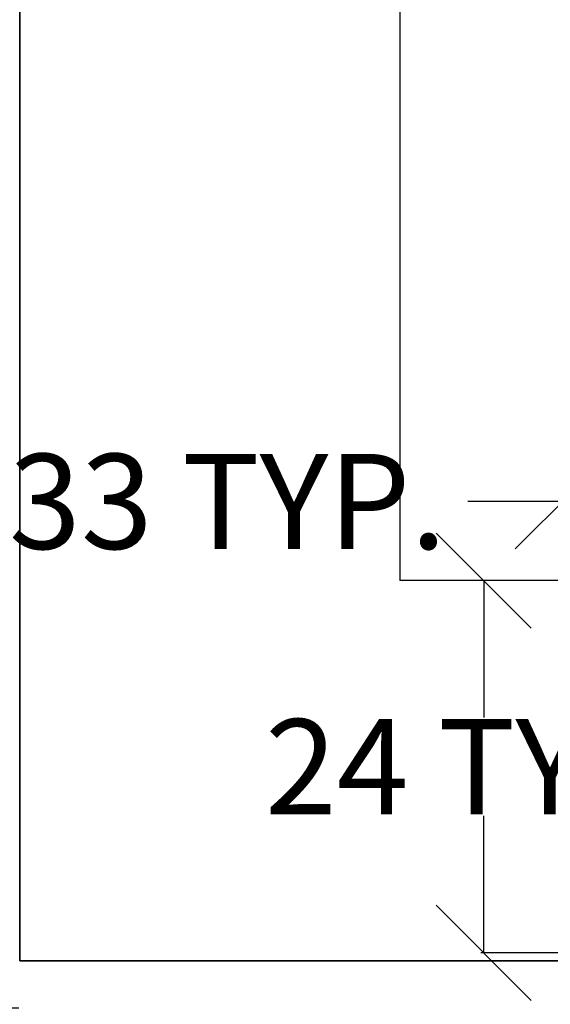
# Model space of a CAD drawing. Units: inches. Extents: x -1198 to -69, y -512 to 437.
# Tile 6 of 50: x -1013 to -979, y 158 to 221. Entities that reach past the tile are written whole.
import ezdxf

# ---------------------------------------------------------------- set-up
doc = ezdxf.new("R2010")
doc.units = ezdxf.units.IN
doc.header["$MEASUREMENT"] = 0
for name, color, linetype, lineweight in [('A-ANNO-DIMS', 2, 'Continuous', 18), ('A-FLOR-CASE', 7, 'Continuous', 25), ('A-WALL', 7, 'Continuous', 35)]:
    doc.layers.add(name, color=color, linetype=linetype, lineweight=lineweight)
doc.styles.get("Standard").update_dxf_attribs({"font": 'arial.ttf'})
doc.dimstyles.get("Standard").update_dxf_attribs({"dimtxt": 6, "dimasz": 6, "dimexe": 0.18, "dimexo": 0.0625, "dimgap": 0.09, "dimtad": 0, "dimtih": 1, "dimtoh": 1, "dimdec": 0, "dimzin": 0, "dimdsep": 46, "dimlunit": 4, "dimtxsty": 'Standard', "dimblk": 'OBLIQUE', "dimcen": 0.09, "dimadec": 0, "dimazin": 0, "dimtfac": 1, "dimtdec": 0, "dimtofl": 0, "dimtmove": 0, "dimatfit": 3, "dimfxl": 1, "dimtolj": 1, "dimtzin": 0, "dimarcsym": 0})

# ---------------------------------------------------------------- blocks, each defined once
blk = doc.blocks.new('COUNTER-L')
at = {"ltscale": 10}
for p in [(0, 96), (49.349, 24)]:
    blk.add_line(p, (0, 24), dxfattribs=at)
blk = doc.blocks.new('_Oblique')
at = {"color": 0, "linetype": 'ByBlock', "lineweight": -2}
blk.add_line((-0.5, -0.5), (0.5, 0.5), dxfattribs=at)
blk = doc.blocks.new('*D50')
at = {"layer": 'A-ANNO-DIMS', "color": 0, "lineweight": -2, "ltscale": 10, "transparency": 16777216}
for p, q in [((-978.462, 190.223), (-984.462, 190.223)), ((-978.462, 185.29), (-978.462, 190.403)), ((-945.163, 190.223), (-978.462, 190.223)), ((-945.163, 185.29), (-945.163, 190.403))]:
    blk.add_line(p, q, dxfattribs=at)
at = {"layer": 'DEFPOINTS', "color": 0, "ltscale": 10, "transparency": 16777216}
for p in [(-978.462, 190.223), (-978.462, 185.228), (-945.163, 185.228)]:
    blk.add_point(p, dxfattribs=at)
at = {"layer": 'A-ANNO-DIMS', "color": 0, "lineweight": -2, "ltscale": 10, "transparency": 16777216, "xscale": 6, "yscale": 6, "zscale": 6, "rotation": 180}
blk.add_blockref('_Oblique', (-978.462, 190.223), dxfattribs=at)
at = {"layer": 'A-ANNO-DIMS', "color": 0, "lineweight": -2, "ltscale": 10, "transparency": 16777216, "xscale": 6, "yscale": 6, "zscale": 6}
blk.add_blockref('_Oblique', (-945.163, 190.223), dxfattribs=at)
at = {"layer": 'A-ANNO-DIMS', "color": 0, "ltscale": 10, "transparency": 16777216, "insert": (-1009.24, 190.223), "char_height": 6, "attachment_point": 5}
blk.add_mtext('\\A1;HOB 33 TYP.', dxfattribs=at)
blk = doc.blocks.new('*D51')
at = {"layer": 'A-ANNO-DIMS', "color": 0, "lineweight": -2, "ltscale": 10, "transparency": 16777216}
for p, q in [((-978.525, 185.228), (-983.637, 185.228)), ((-983.457, 185.228), (-983.457, 176.582)), ((-983.457, 161.727), (-983.457, 170.373)), ((-978.525, 161.727), (-983.637, 161.727))]:
    blk.add_line(p, q, dxfattribs=at)
at = {"layer": 'DEFPOINTS', "color": 0, "ltscale": 10, "transparency": 16777216}
for p in [(-978.462, 185.228), (-983.457, 161.727), (-978.462, 161.727)]:
    blk.add_point(p, dxfattribs=at)
at = {"layer": 'A-ANNO-DIMS', "color": 0, "lineweight": -2, "ltscale": 10, "transparency": 16777216, "xscale": 6, "yscale": 6, "zscale": 6}
for p, rotation in [((-983.457, 185.228), 90), ((-983.457, 161.727), 270)]:
    blk.add_blockref('_Oblique', p, dxfattribs=dict(at, rotation=rotation))
at = {"layer": 'A-ANNO-DIMS', "color": 0, "ltscale": 10, "transparency": 16777216, "insert": (-983.457, 173.478), "char_height": 6, "attachment_point": 5}
blk.add_mtext('\\A1;24 TYP.', dxfattribs=at)
blk = doc.blocks.new('*D80')
at = {"layer": 'A-ANNO-DIMS', "color": 0, "lineweight": -2, "ltscale": 10, "transparency": 16777216}
for p, q in [((-1012.813, 158.228), (-1188.205, 158.228)), ((-1188.025, 158.228), (-1188.025, 140.33)), ((-1188.025, 116.228), (-1188.025, 134.125)), ((-1018.813, 116.228), (-1188.205, 116.228))]:
    blk.add_line(p, q, dxfattribs=at)
at = {"layer": 'DEFPOINTS', "color": 0, "ltscale": 10, "transparency": 16777216}
for p in [(-1188.025, 158.228), (-1012.751, 158.228), (-1018.751, 116.228)]:
    blk.add_point(p, dxfattribs=at)
at = {"layer": 'A-ANNO-DIMS', "color": 0, "lineweight": -2, "ltscale": 10, "transparency": 16777216, "xscale": 6, "yscale": 6, "zscale": 6}
for p, rotation in [((-1188.025, 158.228), 90), ((-1188.025, 116.228), 270)]:
    blk.add_blockref('_Oblique', p, dxfattribs=dict(at, rotation=rotation))
at = {"layer": 'A-ANNO-DIMS', "color": 0, "ltscale": 10, "transparency": 16777216, "insert": (-1188.025, 137.228), "char_height": 6, "attachment_point": 5}
blk.add_mtext('\\A1;42', dxfattribs=at)

msp = doc.modelspace()

# ---------------------------------------------------------------- linework, layer by layer
at = {"layer": 'A-WALL', "ltscale": 10}
for p in [(-1012.7509, 257.2277), (-886.7509, 161.2277)]:
    msp.add_line(p, (-1012.7509, 161.2277), dxfattribs=at)

# ---------------------------------------------------------------- block references
at = {"layer": 'A-FLOR-CASE'}
msp.add_blockref('COUNTER-L', (-988.751, 161.228), dxfattribs=at)

# ---------------------------------------------------------------- dimensions: what is measured, and where the dimension line sits
at = {"layer": 'A-ANNO-DIMS', "ltscale": 10}
for base, p1, p2, angle, text, picture, middle in [((-978.4621, 190.2226), (-945.1627, 185.2277), (-978.4621, 185.2277), 180, 'HOB <> TYP.', '*D50', (-1009.2397, 190.2226)), ((-983.457, 161.7274), (-978.4621, 185.2277), (-978.4621, 161.7274), 270, '<> TYP.', '*D51', (-983.457, 173.4775))]:
    dim = msp.add_linear_dim(base=base, p1=p1, p2=p2, angle=angle, text=text, dimstyle='Standard', override={"dimdec": 0, "dimlfac": 1, "dimrnd": 0, "dimzin": 0, "dimdsep": 46, "dimlunit": 2}, dxfattribs=at)
    dim.commit()
    dim.dimension.update_dxf_attribs({"geometry": picture, "text_midpoint": middle})
dim = msp.add_linear_dim(base=(-1188.0248, 158.2277), p1=(-1018.7509, 116.2277), p2=(-1012.7509, 158.2277), angle=90, dimstyle='Standard', override={"dimdec": 0, "dimlfac": 1, "dimrnd": 0, "dimzin": 0, "dimdsep": 46, "dimlunit": 2}, dxfattribs=at)
dim.commit()
dim.dimension.update_dxf_attribs({"geometry": '*D80', "text_midpoint": (-1188.0248, 137.2277)})

doc.saveas('drawing.dxf')
